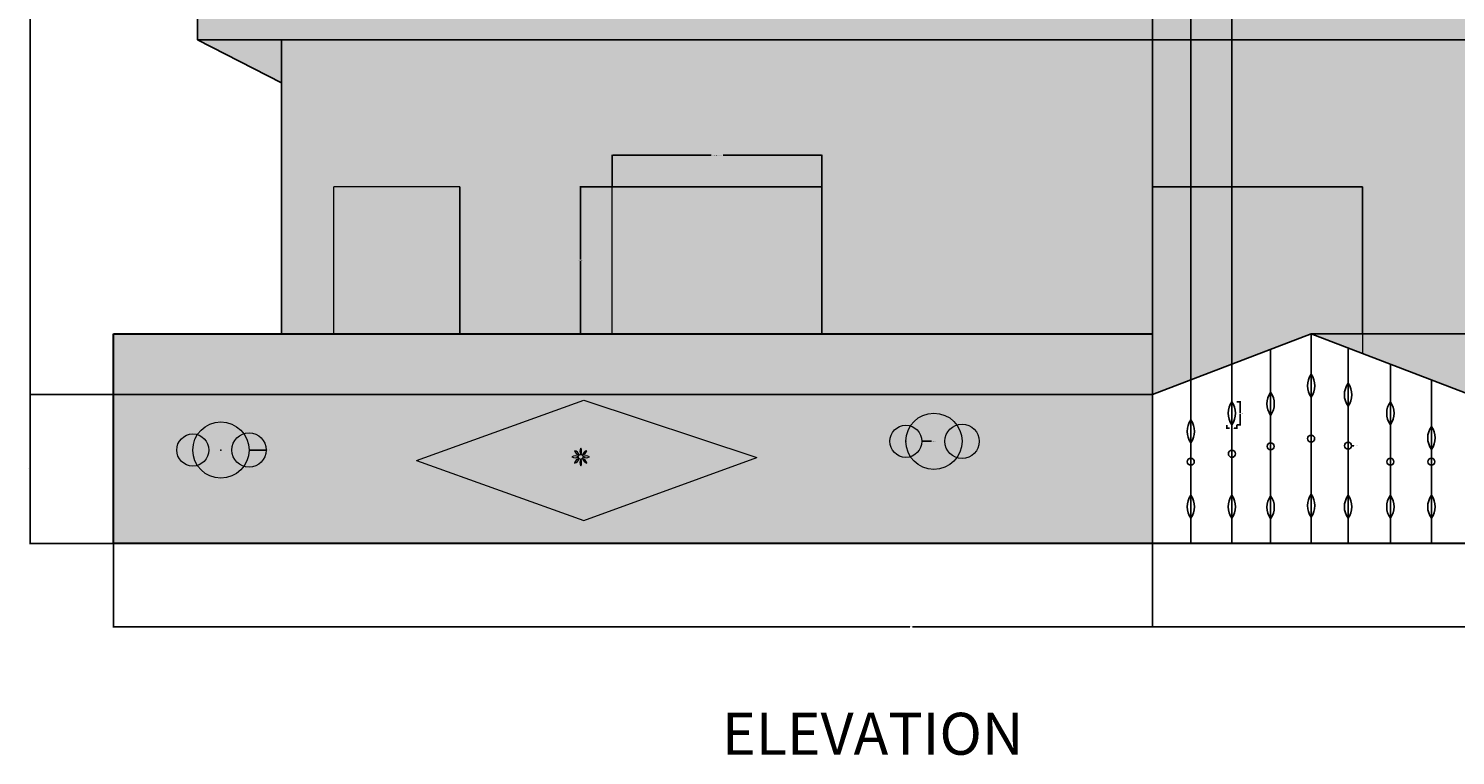
# Model space of a CAD drawing. Units: inches. Extents: x -43 to 1296, y -568 to 542.
# Tile 5 of 14: x -43 to 364, y 128 to 336. Entities that reach past the tile are written whole.
import ezdxf

# ---------------------------------------------------------------- set-up
doc = ezdxf.new("R2010")
doc.units = ezdxf.units.IN
doc.header["$MEASUREMENT"] = 0
for name, color, linetype, lineweight in [('A-ANNO-DIMS', 2, 'Continuous', 18), ('A-ANNO-TEXT', 7, 'Continuous', 18), ('A-DOOR', 3, 'Continuous', 18), ('A-ELEV', 7, 'Continuous', 25), ('A-ELEV-OPEN-PATT', 13, 'Continuous', 13), ('A-ELEV-TRIM', 7, 'Continuous', 18), ('A-ELEV-TRIM-PATT', 4, 'Continuous', 13), ('A-GLAZ-ELEV', 4, 'Continuous', 18), ('A-SITE-GATE', 7, 'Continuous', 25), ('A-SITE-WALL', 7, 'Continuous', 30), ('A-SITE-WALL-PATT', 142, 'Continuous', 13)]:
    doc.layers.add(name, color=color, linetype=linetype, lineweight=lineweight)
doc.layers.add('A-ELEV-BAND-PATT', color=30, linetype='Continuous', lineweight=13, true_color=0xf8991e)
doc.layers.add('A-ELEV-WALL-PATT', color=31, linetype='Continuous', lineweight=13, true_color=0xfecc66)
doc.styles.get("Standard").update_dxf_attribs({"font": 'arial.ttf'})
doc.dimstyles.get("Standard").update_dxf_attribs({"dimtxt": 0.18, "dimasz": 0.18, "dimexe": 0.18, "dimexo": 0.0625, "dimgap": 0.09, "dimtad": 0, "dimtih": 1, "dimtoh": 1, "dimdec": 0, "dimzin": 0, "dimdsep": 46, "dimlunit": 3, "dimtxsty": 'Standard', "dimcen": 0.09, "dimadec": 0, "dimazin": 0, "dimtfac": 1, "dimtdec": 0, "dimtofl": 0, "dimtmove": 0, "dimatfit": 3, "dimfxl": 1, "dimtolj": 1, "dimtzin": 0, "dimarcsym": 0})

# ---------------------------------------------------------------- blocks, each defined once
blk = doc.blocks.new('*U7')
for centre, start, end in [((1.42, 0), 147.6585, 212.3415), ((-1.42, 0), 327.6585, 32.3415)]:
    blk.add_arc(centre, 1.68, start, end)
blk = doc.blocks.new('*U8')
at = {"layer": 'A-ELEV-TRIM', "color": 0, "linetype": 'ByBlock', "lineweight": -2, "transparency": 16777216}
for p, rotation in [((112.78, 213.05), 90), ((113.25, 214.18), 45), ((113.25, 211.91), 135), ((114.38, 211.44), 180), ((115.51, 214.18), 315), ((115.51, 211.91), 225), ((115.98, 213.05), 270)]:
    blk.add_blockref('*U7', p, dxfattribs=dict(at, rotation=rotation))
blk.add_blockref('*U7', (114.38, 214.65), dxfattribs=at)
blk = doc.blocks.new('GATE-PICKET-LEAF')
for centre, start, end in [((5.7, 3.3), 144.6886, 215.3114), ((-3.6, 3.3), 324.6886, 35.3114)]:
    blk.add_arc(centre, 5.7, start, end)
blk = doc.blocks.new('WIN-ELEV-60x42')
for p, q in [((60, 42), (0, 42)), ((0, 0), (0, 42)), ((60, 0), (60, 42))]:
    blk.add_line(p, q)
blk = doc.blocks.new('*D50')
at = {"layer": 'A-ANNO-DIMS', "color": 0, "lineweight": -2, "transparency": 16777216}
for p, q in [((301.95, 228.81), (303.06, 228.81)), ((302.88, 228.63), (302.88, 225.7)), ((302.88, 222.4), (302.88, 225.33)), ((301.95, 222.22), (303.06, 222.22))]:
    blk.add_line(p, q, dxfattribs=at)
at = {"layer": 'A-ANNO-DIMS', "color": 0, "transparency": 16777216}
for points in [[(302.85, 228.63), (302.91, 228.63), (302.88, 228.81)], [(302.85, 222.4), (302.91, 222.4), (302.88, 222.22)]]:
    blk.add_solid(points, dxfattribs=at)
at = {"layer": 'Defpoints', "color": 0, "transparency": 16777216}
for p in [(301.89, 228.81), (302.88, 228.81), (301.89, 222.22)]:
    blk.add_point(p, dxfattribs=at)
at = {"layer": 'A-ANNO-DIMS', "color": 0, "transparency": 16777216, "insert": (302.88, 225.52), "char_height": 0.18, "attachment_point": 5}
blk.add_mtext('\\A1;LEAF 0\'-6 1/2" TYP.', dxfattribs=at)
blk = doc.blocks.new('*D51')
at = {"layer": 'A-ANNO-DIMS', "color": 0, "lineweight": -2, "transparency": 16777216}
for p, q in [((299.09, 222.16), (299.09, 221.05)), ((299.27, 221.23), (299.85, 221.23)), ((301.71, 221.23), (301.13, 221.23)), ((301.89, 222.16), (301.89, 221.05))]:
    blk.add_line(p, q, dxfattribs=at)
at = {"layer": 'A-ANNO-DIMS', "color": 0, "transparency": 16777216}
for points in [[(299.27, 221.26), (299.27, 221.2), (299.09, 221.23)], [(301.71, 221.26), (301.71, 221.2), (301.89, 221.23)]]:
    blk.add_solid(points, dxfattribs=at)
at = {"layer": 'Defpoints', "color": 0, "transparency": 16777216}
for p in [(299.09, 222.22), (301.89, 222.22), (301.89, 221.23)]:
    blk.add_point(p, dxfattribs=at)
at = {"layer": 'A-ANNO-DIMS', "color": 0, "transparency": 16777216, "insert": (300.49, 221.23), "char_height": 0.18, "attachment_point": 5}
blk.add_mtext('\\A1;0\'-3" TYP.', dxfattribs=at)
blk = doc.blocks.new('*D54')
at = {"layer": 'A-ANNO-DIMS', "color": 0, "lineweight": -2, "transparency": 16777216}
for p, q in [((123.34, 290.35), (123.34, 299.47)), ((123.52, 299.29), (151.63, 299.29)), ((183.16, 299.29), (155.06, 299.29)), ((183.34, 290.35), (183.34, 299.47))]:
    blk.add_line(p, q, dxfattribs=at)
at = {"layer": 'A-ANNO-DIMS', "color": 0, "transparency": 16777216}
for points in [[(123.52, 299.32), (123.52, 299.26), (123.34, 299.29)], [(183.16, 299.32), (183.16, 299.26), (183.34, 299.29)]]:
    blk.add_solid(points, dxfattribs=at)
at = {"layer": 'Defpoints', "color": 0, "transparency": 16777216}
for p in [(183.34, 299.29), (123.34, 290.29), (183.34, 290.29)]:
    blk.add_point(p, dxfattribs=at)
at = {"layer": 'A-ANNO-DIMS', "color": 0, "transparency": 16777216, "insert": (153.34, 299.29), "char_height": 0.18, "attachment_point": 5}
blk.add_mtext('\\A1;LOWER WINDOW 5\'-0" TYP.', dxfattribs=at)
blk = doc.blocks.new('*D55')
at = {"layer": 'A-ANNO-DIMS', "color": 0, "lineweight": -2, "transparency": 16777216}
for p, q in [((123.28, 290.29), (114.16, 290.29)), ((114.34, 290.11), (114.34, 269.47)), ((114.34, 248.47), (114.34, 269.11)), ((123.28, 248.29), (114.16, 248.29))]:
    blk.add_line(p, q, dxfattribs=at)
at = {"layer": 'A-ANNO-DIMS', "color": 0, "transparency": 16777216}
for points in [[(114.31, 290.11), (114.37, 290.11), (114.34, 290.29)], [(114.31, 248.47), (114.37, 248.47), (114.34, 248.29)]]:
    blk.add_solid(points, dxfattribs=at)
at = {"layer": 'Defpoints', "color": 0, "transparency": 16777216}
for p in [(114.34, 290.29), (123.34, 290.29), (123.34, 248.29)]:
    blk.add_point(p, dxfattribs=at)
at = {"layer": 'A-ANNO-DIMS', "color": 0, "transparency": 16777216, "insert": (114.34, 269.29), "char_height": 0.18, "attachment_point": 5}
blk.add_mtext('\\A1;3\'-6" TYP.', dxfattribs=at)
blk = doc.blocks.new('*D60')
at = {"layer": 'A-ANNO-DIMS', "color": 0, "lineweight": -2, "transparency": 16777216}
for p, q in [((-19.16, 188.23), (-19.16, 164.31)), ((436.84, 188.23), (436.84, 164.31)), ((-18.98, 164.49), (208.44, 164.49)), ((436.66, 164.49), (209.24, 164.49))]:
    blk.add_line(p, q, dxfattribs=at)
at = {"layer": 'A-ANNO-DIMS', "color": 0, "transparency": 16777216}
for points in [[(-18.98, 164.52), (-18.98, 164.46), (-19.16, 164.49)], [(436.66, 164.52), (436.66, 164.46), (436.84, 164.49)]]:
    blk.add_solid(points, dxfattribs=at)
at = {"layer": 'Defpoints', "color": 0, "transparency": 16777216}
for p in [(-19.16, 188.29), (436.84, 188.29), (436.84, 164.49)]:
    blk.add_point(p, dxfattribs=at)
at = {"layer": 'A-ANNO-DIMS', "color": 0, "transparency": 16777216, "insert": (208.84, 164.49), "char_height": 0.18, "attachment_point": 5}
blk.add_mtext('\\A1;38\'-0"', dxfattribs=at)
blk = doc.blocks.new('*D61')
at = {"layer": 'A-ANNO-DIMS', "color": 0, "lineweight": -2, "transparency": 16777216}
for p, q in [((4.78, 518.29), (-43.14, 518.29)), ((-42.96, 518.11), (-42.96, 353.47)), ((-42.96, 188.47), (-42.96, 353.11)), ((-19.22, 188.29), (-43.14, 188.29))]:
    blk.add_line(p, q, dxfattribs=at)
at = {"layer": 'A-ANNO-DIMS', "color": 0, "transparency": 16777216}
for points in [[(-42.99, 518.11), (-42.93, 518.11), (-42.96, 518.29)], [(-42.99, 188.47), (-42.93, 188.47), (-42.96, 188.29)]]:
    blk.add_solid(points, dxfattribs=at)
at = {"layer": 'Defpoints', "color": 0, "transparency": 16777216}
for p in [(-42.96, 518.29), (4.84, 518.29), (-19.16, 188.29)]:
    blk.add_point(p, dxfattribs=at)
at = {"layer": 'A-ANNO-DIMS', "color": 0, "transparency": 16777216, "insert": (-42.96, 353.29), "char_height": 0.18, "attachment_point": 5}
blk.add_mtext('\\A1;27\'-6"', dxfattribs=at)
blk = doc.blocks.new('*D67')
at = {"layer": 'A-ANNO-DIMS', "color": 0, "lineweight": -2, "transparency": 16777216}
for p, q in [((277.84, 188.23), (277.84, 164.31)), ((368.43, 188.23), (368.43, 164.31)), ((278.02, 164.49), (322.6, 164.49)), ((368.25, 164.49), (323.68, 164.49))]:
    blk.add_line(p, q, dxfattribs=at)
at = {"layer": 'A-ANNO-DIMS', "color": 0, "transparency": 16777216}
for points in [[(278.02, 164.52), (278.02, 164.46), (277.84, 164.49)], [(368.25, 164.52), (368.25, 164.46), (368.43, 164.49)]]:
    blk.add_solid(points, dxfattribs=at)
at = {"layer": 'Defpoints', "color": 0, "transparency": 16777216}
for p in [(277.84, 188.29), (368.43, 188.29), (368.43, 164.49)]:
    blk.add_point(p, dxfattribs=at)
at = {"layer": 'A-ANNO-DIMS', "color": 0, "transparency": 16777216, "insert": (323.14, 164.49), "char_height": 0.18, "attachment_point": 5}
blk.add_mtext('\\A1;7\'-6 1/2"', dxfattribs=at)
blk = doc.blocks.new('*D68')
at = {"layer": 'A-ANNO-DIMS', "color": 0, "lineweight": -2, "transparency": 16777216}
for p, q in [((277.78, 230.87), (-43.14, 230.87)), ((-42.96, 230.69), (-42.96, 209.77)), ((-42.96, 188.47), (-42.96, 209.4)), ((277.78, 188.29), (-43.14, 188.29))]:
    blk.add_line(p, q, dxfattribs=at)
at = {"layer": 'A-ANNO-DIMS', "color": 0, "transparency": 16777216}
for points in [[(-42.99, 230.69), (-42.93, 230.69), (-42.96, 230.87)], [(-42.99, 188.47), (-42.93, 188.47), (-42.96, 188.29)]]:
    blk.add_solid(points, dxfattribs=at)
at = {"layer": 'Defpoints', "color": 0, "transparency": 16777216}
for p in [(277.84, 230.87), (-42.96, 188.29), (277.84, 188.29)]:
    blk.add_point(p, dxfattribs=at)
at = {"layer": 'A-ANNO-DIMS', "color": 0, "transparency": 16777216, "insert": (-42.96, 209.58), "char_height": 0.18, "attachment_point": 5}
blk.add_mtext('\\A1;3\'-6 1/2"', dxfattribs=at)
blk = doc.blocks.new('*D69')
at = {"layer": 'A-ANNO-DIMS', "color": 0, "lineweight": -2, "transparency": 16777216}
for p, q in [((323.2, 248.29), (460.82, 248.29)), ((460.64, 248.11), (460.64, 218.47)), ((460.64, 188.47), (460.64, 218.11)), ((368.5, 188.29), (460.82, 188.29))]:
    blk.add_line(p, q, dxfattribs=at)
at = {"layer": 'A-ANNO-DIMS', "color": 0, "transparency": 16777216}
for points in [[(460.61, 248.11), (460.67, 248.11), (460.64, 248.29)], [(460.61, 188.47), (460.67, 188.47), (460.64, 188.29)]]:
    blk.add_solid(points, dxfattribs=at)
at = {"layer": 'Defpoints', "color": 0, "transparency": 16777216}
for p in [(323.14, 248.29), (368.43, 188.29), (460.64, 188.29)]:
    blk.add_point(p, dxfattribs=at)
at = {"layer": 'A-ANNO-DIMS', "color": 0, "transparency": 16777216, "insert": (460.64, 218.29), "char_height": 0.18, "attachment_point": 5}
blk.add_mtext('\\A1;5\'-0"', dxfattribs=at)
blk = doc.blocks.new('*D70')
at = {"layer": 'A-ANNO-DIMS', "color": 0, "lineweight": -2, "transparency": 16777216}
for p, q in [((277.84, 188.35), (277.84, 542.27)), ((278.02, 542.09), (282.89, 542.09)), ((288.57, 542.09), (283.69, 542.09)), ((288.75, 188.35), (288.75, 542.27))]:
    blk.add_line(p, q, dxfattribs=at)
at = {"layer": 'A-ANNO-DIMS', "color": 0, "transparency": 16777216}
for points in [[(278.02, 542.12), (278.02, 542.06), (277.84, 542.09)], [(288.57, 542.12), (288.57, 542.06), (288.75, 542.09)]]:
    blk.add_solid(points, dxfattribs=at)
at = {"layer": 'Defpoints', "color": 0, "transparency": 16777216}
for p in [(288.75, 542.09), (277.84, 188.29), (288.75, 188.29)]:
    blk.add_point(p, dxfattribs=at)
at = {"layer": 'A-ANNO-DIMS', "color": 0, "transparency": 16777216, "insert": (283.29, 542.09), "char_height": 0.18, "attachment_point": 5}
blk.add_mtext('\\A1;0\'-11"', dxfattribs=at)
blk = doc.blocks.new('*D71')
at = {"layer": 'A-ANNO-DIMS', "color": 0, "lineweight": -2, "transparency": 16777216}
for p, q in [((288.75, 235.13), (288.75, 542.27)), ((288.93, 542.09), (294.01, 542.09)), ((300.31, 542.09), (295.23, 542.09)), ((300.49, 239.65), (300.49, 542.27))]:
    blk.add_line(p, q, dxfattribs=at)
at = {"layer": 'A-ANNO-DIMS', "color": 0, "transparency": 16777216}
for points in [[(288.93, 542.12), (288.93, 542.06), (288.75, 542.09)], [(300.31, 542.12), (300.31, 542.06), (300.49, 542.09)]]:
    blk.add_solid(points, dxfattribs=at)
at = {"layer": 'Defpoints', "color": 0, "transparency": 16777216}
for p in [(300.49, 542.09), (300.49, 239.58), (288.75, 235.07)]:
    blk.add_point(p, dxfattribs=at)
at = {"layer": 'A-ANNO-DIMS', "color": 0, "transparency": 16777216, "insert": (294.62, 542.09), "char_height": 0.18, "attachment_point": 5}
blk.add_mtext('\\A1;0\'-11 1/2"', dxfattribs=at)
blk = doc.blocks.new('*D98')
at = {"layer": 'A-ANNO-DIMS', "color": 0, "lineweight": -2, "transparency": 16777216}
for p, q in [((333.62, 216.26), (333.8, 216.26)), ((333.71, 216.17), (333.71, 216.35)), ((335.31, 216.25), (334.89, 216.25))]:
    blk.add_line(p, q, dxfattribs=at)
at = {"layer": 'A-ANNO-DIMS', "color": 0, "transparency": 16777216}
blk.add_solid([(334.89, 216.28), (334.89, 216.22), (334.71, 216.25)], dxfattribs=at)
at = {"layer": 'Defpoints', "color": 0, "transparency": 16777216}
for p in [(332.71, 216.27), (334.71, 216.25)]:
    blk.add_point(p, dxfattribs=at)
at = {"layer": 'A-ANNO-DIMS', "color": 0, "transparency": 16777216, "insert": (335.93, 216.25), "char_height": 0.18, "attachment_point": 5}
blk.add_mtext('\\A1;7X ∅0\'-2"', dxfattribs=at)
blk = doc.blocks.new('*D99')
at = {"layer": 'A-ANNO-DIMS', "color": 0, "lineweight": -2, "transparency": 16777216}
for p, q in [((11.46, 215.02), (11.64, 215.02)), ((11.55, 214.93), (11.55, 215.11)), ((24.41, 215.02), (19.77, 215.02))]:
    blk.add_line(p, q, dxfattribs=at)
at = {"layer": 'A-ANNO-DIMS', "color": 0, "transparency": 16777216}
blk.add_solid([(19.77, 215.05), (19.77, 214.99), (19.59, 215.02)], dxfattribs=at)
at = {"layer": 'Defpoints', "color": 0, "transparency": 16777216}
for p in [(3.51, 215.02), (19.59, 215.02)]:
    blk.add_point(p, dxfattribs=at)
at = {"layer": 'A-ANNO-DIMS', "color": 0, "transparency": 16777216, "insert": (25.03, 215.02), "char_height": 0.18, "attachment_point": 5}
blk.add_mtext('\\A1;3X ∅1\'-4"', dxfattribs=at)
blk = doc.blocks.new('*D101')
at = {"layer": 'A-ANNO-DIMS', "color": 0, "lineweight": -2, "transparency": 16777216}
for p, q in [((207.21, 217.51), (207.39, 217.51)), ((207.3, 217.42), (207.3, 217.6)), ((214.65, 217.51), (212.07, 217.51))]:
    blk.add_line(p, q, dxfattribs=at)
at = {"layer": 'A-ANNO-DIMS', "color": 0, "transparency": 16777216}
blk.add_solid([(212.07, 217.54), (212.07, 217.48), (211.89, 217.51)], dxfattribs=at)
at = {"layer": 'Defpoints', "color": 0, "transparency": 16777216}
for p in [(202.71, 217.51), (211.89, 217.51)]:
    blk.add_point(p, dxfattribs=at)
at = {"layer": 'A-ANNO-DIMS', "color": 0, "transparency": 16777216, "insert": (215.26, 217.51), "char_height": 0.18, "attachment_point": 5}
blk.add_mtext('\\A1;3X ∅0\'-9"', dxfattribs=at)

msp = doc.modelspace()

# ---------------------------------------------------------------- hatches: boundary and pattern name
at = {"layer": 'A-ELEV-BAND-PATT'}
h = msp.add_hatch(color=256, dxfattribs=at)
h.dxf.hatch_style = 1
h.paths.add_polyline_path([(28.84, 332.29), (4.84, 332.29), (28.84, 320)])
h.paths.add_polyline_path([(412.84, 332.29), (388.84, 332.29), (388.84, 323.84)])
h.paths.add_polyline_path([(1184.13, 416.59), (824.13, 416.59), (824.13, 410.59), (1184.13, 410.59)])
h.paths.add_polyline_path([(1184.13, 272.59), (824.13, 272.59), (824.13, 266.59), (1184.13, 266.59)])
h = msp.add_hatch(color=256, dxfattribs=at)
h.dxf.hatch_style = 1
h.paths.add_polyline_path([(412.84, 374.29), (4.84, 374.29), (4.84, 332.29), (412.84, 332.29)])
h.paths.add_polyline_path([(222.28, 353.73, -0.197856), (210.28, 353.73, -0.131652), (209.89, 352.27, -0.197856), (220.28, 346.27, -0.197856), (209.89, 352.27, -0.131652), (208.82, 351.2, -0.197856), (214.82, 340.81, -0.197856), (208.82, 351.2, -0.131652), (207.36, 350.81, -0.197856), (207.36, 338.81, -0.197856), (207.36, 350.81, -0.131652), (205.9, 351.2, -0.197856), (199.9, 340.81, -0.197856), (205.9, 351.2, -0.131652), (204.83, 352.27, -0.197856), (194.44, 346.27, -0.197856), (204.83, 352.27, -0.131652), (204.44, 353.73, -0.197856), (192.44, 353.73, -0.197856), (204.44, 353.73, -0.131652), (204.83, 355.19, -0.197856), (194.44, 361.19, -0.197856), (204.83, 355.19, -0.131652), (205.9, 356.25, -0.197856), (199.9, 366.65, -0.197856), (205.9, 356.25, -0.131652), (207.36, 356.65, -0.197856), (207.36, 368.65, -0.197856), (207.36, 356.65, -0.131652), (208.82, 356.25, -0.197856), (214.82, 366.65, -0.197856), (208.82, 356.25, -0.131652), (209.89, 355.19, -0.197856), (220.28, 361.19, -0.197856), (209.89, 355.19, -0.131652), (210.28, 353.73, -0.197856)], flags=16)
h.paths.add_polyline_path([(263.61, 353.73, -0.197856), (275.61, 353.73, -0.131652), (276, 355.19, -0.197856), (265.61, 361.19, -0.197856), (276, 355.19, -0.131652), (277.07, 356.25, -0.197856), (271.07, 366.65, -0.197856), (277.07, 356.25, -0.131652), (278.53, 356.65, -0.197856), (278.53, 368.65, -0.197856), (278.53, 356.65, -0.131652), (279.99, 356.25, -0.197856), (285.99, 366.65, -0.197856), (279.99, 356.25, -0.131652), (281.06, 355.19, -0.197856), (291.45, 361.19, -0.197856), (281.06, 355.19, -0.131652), (281.45, 353.73, -0.197856), (293.45, 353.73, -0.197856), (281.45, 353.73, -0.131652), (281.06, 352.27, -0.197856), (291.45, 346.27, -0.197856), (281.06, 352.27, -0.131652), (279.99, 351.2, -0.197856), (285.99, 340.81, -0.197856), (279.99, 351.2, -0.131652), (278.53, 350.81, -0.197856), (278.53, 338.81, -0.197856), (278.53, 350.81, -0.131652), (277.07, 351.2, -0.197856), (271.07, 340.81, -0.197856), (277.07, 351.2, -0.131652), (276, 352.27, -0.197856), (265.61, 346.27, -0.197856), (276, 352.27, -0.131652), (275.61, 353.73, -0.197856)], flags=16)
h.paths.add_polyline_path([(330.52, 353.73, -0.197856), (342.52, 353.73, -0.131652), (342.91, 355.19, -0.197856), (332.52, 361.19, -0.197856), (342.91, 355.19, -0.131652), (343.98, 356.25, -0.197856), (337.98, 366.65, -0.197856), (343.98, 356.25, -0.131652), (345.44, 356.65, -0.197856), (345.44, 368.65, -0.197856), (345.44, 356.65, -0.131652), (346.9, 356.25, -0.197856), (352.9, 366.65, -0.197856), (346.9, 356.25, -0.131652), (347.97, 355.19, -0.197856), (358.36, 361.19, -0.197856), (347.97, 355.19, -0.131652), (348.36, 353.73, -0.197856), (360.36, 353.73, -0.197856), (348.36, 353.73, -0.131652), (347.97, 352.27, -0.197856), (358.36, 346.27, -0.197856), (347.97, 352.27, -0.131652), (346.9, 351.2, -0.197856), (352.9, 340.81, -0.197856), (346.9, 351.2, -0.131652), (345.44, 350.81, -0.197856), (345.44, 338.81, -0.197856), (345.44, 350.81, -0.131652), (343.98, 351.2, -0.197856), (337.98, 340.81, -0.197856), (343.98, 351.2, -0.131652), (342.91, 352.27, -0.197856), (332.52, 346.27, -0.197856), (342.91, 352.27, -0.131652), (342.52, 353.73, -0.197856)], flags=16)
h.paths.add_polyline_path([(148.25, 353.73, -0.197856), (136.25, 353.73, -0.131652), (135.85, 352.27, -0.197856), (146.25, 346.27, -0.197856), (135.85, 352.27, -0.131652), (134.79, 351.2, -0.197856), (140.79, 340.81, -0.197856), (134.79, 351.2, -0.131652), (133.33, 350.81, -0.197856), (133.33, 338.81, -0.197856), (133.33, 350.81, -0.131652), (131.87, 351.2, -0.197856), (125.87, 340.81, -0.197856), (131.87, 351.2, -0.131652), (130.8, 352.27, -0.197856), (120.41, 346.27, -0.197856), (130.8, 352.27, -0.131652), (130.41, 353.73, -0.197856), (118.41, 353.73, -0.197856), (130.41, 353.73, -0.131652), (130.8, 355.19, -0.197856), (120.41, 361.19, -0.197856), (130.8, 355.19, -0.131652), (131.87, 356.25, -0.197856), (125.87, 366.65, -0.197856), (131.87, 356.25, -0.131652), (133.33, 356.65, -0.197856), (133.33, 368.65, -0.197856), (133.33, 356.65, -0.131652), (134.79, 356.25, -0.197856), (140.79, 366.65, -0.197856), (134.79, 356.25, -0.131652), (135.85, 355.19, -0.197856), (146.25, 361.19, -0.197856), (135.85, 355.19, -0.131652), (136.25, 353.73, -0.197856)], flags=16)
h.paths.add_polyline_path([(80.61, 353.73, -0.197856), (68.61, 353.73, -0.131652), (68.22, 352.27, -0.197856), (78.61, 346.27, -0.197856), (68.22, 352.27, -0.131652), (67.15, 351.2, -0.197856), (73.15, 340.81, -0.197856), (67.15, 351.2, -0.131652), (65.69, 350.81, -0.197856), (65.69, 338.81, -0.197856), (65.69, 350.81, -0.131652), (64.23, 351.2, -0.197856), (58.23, 340.81, -0.197856), (64.23, 351.2, -0.131652), (63.16, 352.27, -0.197856), (52.77, 346.27, -0.197856), (63.16, 352.27, -0.131652), (62.77, 353.73, -0.197856), (50.77, 353.73, -0.197856), (62.77, 353.73, -0.131652), (63.16, 355.19, -0.197856), (52.77, 361.19, -0.197856), (63.16, 355.19, -0.131652), (64.23, 356.25, -0.197856), (58.23, 366.65, -0.197856), (64.23, 356.25, -0.131652), (65.69, 356.65, -0.197856), (65.69, 368.65, -0.197856), (65.69, 356.65, -0.131652), (67.15, 356.25, -0.197856), (73.15, 366.65, -0.197856), (67.15, 356.25, -0.131652), (68.22, 355.19, -0.197856), (78.61, 361.19, -0.197856), (68.22, 355.19, -0.131652), (68.61, 353.73, -0.197856)], flags=16)
at = {"layer": 'A-ELEV-OPEN-PATT'}
h = msp.add_hatch(color=256, dxfattribs=at)
h.dxf.hatch_style = 1
h.paths.add_polyline_path([(79.84, 434.29), (43.84, 434.29), (43.84, 374.29), (79.84, 374.29)])
h.paths.add_polyline_path([(183.34, 434.29), (123.34, 434.29), (123.34, 386.29), (183.34, 386.29)])
h.paths.add_polyline_path([(337.84, 434.29), (277.84, 434.29), (277.84, 386.29), (337.84, 386.29)])
h.paths.add_polyline_path([(79.84, 290.29), (43.84, 290.29), (43.84, 248.29), (79.84, 248.29)])
h.paths.add_polyline_path([(183.34, 290.29), (123.34, 290.29), (123.34, 248.29), (183.34, 248.29)])
h.paths.add_polyline_path([(337.84, 290.29), (277.84, 290.29), (277.84, 248.29), (277.84, 230.87), (323.14, 248.29), (337.84, 242.64), (337.84, 248.29)])
h.paths.add_polyline_path([(1016.13, 374.59), (980.13, 374.59), (980.13, 290.59), (1016.13, 290.59)])
h.paths.add_polyline_path([(1016.13, 230.59), (980.13, 230.59), (980.13, 146.59), (1016.13, 146.59)])
h.paths.add_polyline_path([(833.13, 374.59), (824.13, 374.59), (824.13, 326.59), (833.13, 326.59)])
h.paths.add_polyline_path([(833.13, 230.59), (824.13, 230.59), (824.13, 182.59), (833.13, 182.59)])
at = {"layer": 'A-ELEV-TRIM-PATT'}
h = msp.add_hatch(color=256, dxfattribs=at)
h.dxf.hatch_style = 1
h.paths.add_polyline_path([(164.68, 212.9), (115.24, 229.23), (67.47, 212.06), (115.24, 194.9)])
h.paths.add_polyline_path([(116.88, 213.05, -0.289973), (115.08, 213.05, -0.198912), (114.88, 212.55, -0.289973), (116.15, 211.28, -0.289973), (114.88, 212.55, -0.198912), (114.38, 212.34, -0.289973), (114.38, 210.55, -0.289973), (114.38, 212.34, -0.198912), (113.88, 212.55, -0.289973), (112.61, 211.28, -0.289973), (113.88, 212.55, -0.198912), (113.68, 213.05, -0.289973), (111.88, 213.05, -0.289973), (113.68, 213.05, -0.198912), (113.88, 213.54, -0.289973), (112.61, 214.81, -0.289973), (113.88, 213.54, -0.198912), (114.38, 213.75, -0.289973), (114.38, 215.55, -0.289973), (114.38, 213.75, -0.198912), (114.88, 213.54, -0.289973), (116.15, 214.81, -0.289973), (114.88, 213.54, -0.198912), (115.08, 213.05, -0.289973)], flags=16)
h.paths.add_polyline_path([(218.46, 217.51, -0.325786), (221.87, 222.19, 0.526984), (208.61, 221.91, -0.331674), (211.89, 217.51, -0.331674), (208.61, 213.11, 0.526984), (221.87, 212.82, -0.325786)])
h.paths.add_polyline_path([(404.4, 217.51, -0.325786), (407.82, 222.19, 0.526984), (394.56, 221.91, -0.331674), (397.84, 217.51, -0.331674), (394.56, 213.11, 0.526984), (407.82, 212.82, -0.325786)])
h.paths.add_polyline_path([(14.67, 215.02, -0.325786), (18.08, 219.7, 0.526984), (4.82, 219.42, -0.331674), (8.11, 215.02, -0.331674), (4.82, 210.62, 0.526984), (18.08, 210.34, -0.325786)])
h = msp.add_hatch(color=256, dxfattribs=at)
h.dxf.hatch_style = 1
h.paths.add_polyline_path([(115.08, 213.05, 1), (113.68, 213.05, 1)])
h.paths.add_polyline_path([(114.38, 215.55, 0.289973), (114.38, 213.75, 0.289973)])
h.paths.add_polyline_path([(112.61, 214.81, 0.289973), (113.88, 213.54, 0.289973)])
h.paths.add_polyline_path([(113.68, 213.05, 0.289973), (111.88, 213.05, 0.289973)])
h.paths.add_polyline_path([(113.88, 212.55, 0.289973), (112.61, 211.28, 0.289973)])
h.paths.add_polyline_path([(114.38, 212.34, 0.289973), (114.38, 210.55, 0.289973)])
h.paths.add_polyline_path([(114.88, 212.55, 0.289973), (116.15, 211.28, 0.289973)])
h.paths.add_polyline_path([(115.08, 213.05, 0.289973), (116.88, 213.05, 0.289973)])
h.paths.add_polyline_path([(116.15, 214.81, 0.289973), (114.88, 213.54, 0.289973)])
h.paths.add_polyline_path([(8.11, 215.02, 0.331674), (4.82, 219.42, 0.145907), (3.51, 215.02, 0.145907), (4.82, 210.62, 0.331674)])
h.paths.add_polyline_path([(19.59, 215.02, 0.156779), (18.08, 219.7, 0.325786), (14.67, 215.02, 0.325786), (18.08, 210.34, 0.156779)])
h.paths.add_polyline_path([(18.08, 219.7, -0.156779), (19.59, 215.02, -0.156779), (18.08, 210.34, 0.508539), (24.51, 215.02, 0.508539)])
h.paths.add_polyline_path([(4.82, 219.42, 0.501869), (-1.08, 215.02, 0.501869), (4.82, 210.62, -0.145907), (3.51, 215.02, -0.145907)])
h.paths.add_polyline_path([(228.3, 217.51, 0.508539), (221.87, 222.19, -0.156779), (223.38, 217.51, -0.156779), (221.87, 212.82, 0.508539)])
h.paths.add_polyline_path([(223.38, 217.51, 0.156779), (221.87, 222.19, 0.325786), (218.46, 217.51, 0.325786), (221.87, 212.82, 0.156779)])
h.paths.add_polyline_path([(211.89, 217.51, 0.331674), (208.61, 221.91, 0.145907), (207.3, 217.51, 0.145907), (208.61, 213.11, 0.331674)])
h.paths.add_polyline_path([(208.61, 221.91, 0.501869), (202.71, 217.51, 0.501869), (208.61, 213.11, -0.145907), (207.3, 217.51, -0.145907)])
h.paths.add_polyline_path([(407.82, 222.19, -0.156779), (409.32, 217.51, -0.156779), (407.82, 212.82, 0.508539), (414.24, 217.51, 0.508539)])
h.paths.add_polyline_path([(393.25, 217.51, -0.145907), (394.56, 221.91, 0.501869), (388.65, 217.51, 0.501869), (394.56, 213.11, -0.145907)])
h.paths.add_polyline_path([(397.84, 217.51, 0.331674), (394.56, 221.91, 0.145907), (393.25, 217.51, 0.145907), (394.56, 213.11, 0.331674)])
h.paths.add_polyline_path([(409.32, 217.51, 0.156779), (407.82, 222.19, 0.325786), (404.4, 217.51, 0.325786), (407.82, 212.82, 0.156779)])
at = {"layer": 'A-ELEV-WALL-PATT'}
h = msp.add_hatch(color=256, dxfattribs=at)
h.dxf.hatch_style = 1
h.paths.add_polyline_path([(388.84, 332.29), (28.84, 332.29), (28.84, 248.29), (43.84, 248.29), (43.84, 290.29), (79.84, 290.29), (79.84, 248.29), (123.34, 248.29), (123.34, 290.29), (183.34, 290.29), (183.34, 248.29), (277.84, 248.29), (277.84, 290.29), (337.84, 290.29), (337.84, 248.29), (337.84, 242.64), (368.43, 230.87), (368.43, 248.29), (388.84, 248.29)])
at = {"layer": 'A-SITE-WALL-PATT'}
h = msp.add_hatch(color=256, dxfattribs=at)
h.dxf.hatch_style = 1
h.paths.add_polyline_path([(277.84, 248.29), (-19.16, 248.29), (-19.16, 188.29), (28.84, 188.29), (277.84, 188.29)])
h.paths.add_polyline_path([(115.24, 229.23), (164.68, 212.9), (115.24, 194.9), (67.47, 212.06)], flags=16)
h.paths.add_polyline_path([(112.61, 214.81, -0.289973), (113.88, 213.54, -0.198912), (114.38, 213.75, -0.289973), (114.38, 215.55, -0.289973), (114.38, 213.75, -0.198912), (114.88, 213.54, -0.289973), (116.15, 214.81, -0.289973), (114.88, 213.54, -0.198912), (115.08, 213.05, -0.289973), (116.88, 213.05, -0.289973), (115.08, 213.05, -0.198912), (114.88, 212.55, -0.289973), (116.15, 211.28, -0.289973), (114.88, 212.55, -0.198912), (114.38, 212.34, -0.289973), (114.38, 210.55, -0.289973), (114.38, 212.34, -0.198912), (113.88, 212.55, -0.289973), (112.61, 211.28, -0.289973), (113.88, 212.55, -0.198912), (113.68, 213.05, -0.289973), (111.88, 213.05, -0.289973), (113.68, 213.05, -0.198912), (113.88, 213.54, -0.289973)], flags=0)
h.paths.add_polyline_path([(24.51, 215.02, -0.508539), (18.08, 210.34, -0.526984), (4.82, 210.62, -0.501869), (-1.08, 215.02, -0.501869), (4.82, 219.42, -0.526984), (18.08, 219.7, -0.508539)], flags=16)
h.paths.add_polyline_path([(208.61, 221.91, -0.526984), (221.87, 222.19, -0.508539), (228.3, 217.51, -0.508539), (221.87, 212.82, -0.526984), (208.61, 213.11, -0.501869), (202.71, 217.51, -0.501869)], flags=16)
h.paths.add_polyline_path([(436.84, 248.29), (368.43, 248.29), (368.43, 188.29), (388.84, 188.29), (436.84, 188.29)])
h.paths.add_polyline_path([(394.56, 221.91, -0.526984), (407.82, 222.19, -0.508539), (414.24, 217.51, -0.508539), (407.82, 212.82, -0.526984), (394.56, 213.11, -0.501869), (388.65, 217.51, -0.501869)], flags=16)

# ---------------------------------------------------------------- linework, layer by layer
at = {"layer": 'A-DOOR'}
for p, q in [((43.84, 248.29), (43.84, 290.29)), ((79.84, 290.29), (43.84, 290.29)), ((79.84, 248.29), (79.84, 290.29))]:
    msp.add_line(p, q, dxfattribs=at)
for points in [[(43.84, 248.29), (43.84, 290.29)], [(79.84, 290.29), (79.84, 248.29)]]:
    msp.add_lwpolyline(points, dxfattribs=at)
at = {"layer": 'A-ELEV'}
for p, q in [((4.84, 332.29), (4.84, 374.29)), ((412.84, 332.29), (4.84, 332.29)), ((4.84, 332.29), (28.84, 320)), ((28.84, 248.29), (28.84, 332.29))]:
    msp.add_line(p, q, dxfattribs=at)
at = {"layer": 'A-ELEV-TRIM'}
for p, q in [((67.47, 212.06), (115.24, 229.23)), ((115.24, 229.23), (164.68, 212.9)), ((115.24, 194.9), (164.68, 212.9)), ((67.47, 212.06), (115.24, 194.9))]:
    msp.add_line(p, q, dxfattribs=at)
for centre, radius in [((215.34, 217.51), 8.04), ((11.55, 215.02), 8.04), ((207.3, 217.51), 4.59), ((223.38, 217.51), 4.92), ((3.51, 215.02), 4.59), ((19.59, 215.02), 4.92), ((114.38, 213.05), 0.703)]:
    msp.add_circle(centre, radius, dxfattribs=at)
at = {"layer": 'A-GLAZ-ELEV'}
msp.add_line((337.84, 248.29), (337.84, 242.64), dxfattribs=at)
for points in [[(123.34, 248.29), (123.34, 290.29), (183.34, 290.29), (183.34, 248.29)], [(277.84, 248.29), (277.84, 290.29), (337.84, 290.29), (337.84, 248.29)]]:
    msp.add_lwpolyline(points, dxfattribs=at)
at = {"layer": 'A-SITE-GATE'}
for p, q in [((277.84, 248.29), (277.84, 188.29)), ((323.14, 248.29), (277.84, 230.87)), ((323.14, 248.29), (368.43, 230.87)), ((323.14, 248.29), (323.14, 188.29)), ((311.57, 243.84), (311.57, 188.29)), ((333.71, 244.23), (333.71, 188.29)), ((300.49, 239.58), (300.49, 188.29)), ((345.79, 239.58), (345.79, 188.29)), ((288.75, 235.07), (288.75, 188.29)), ((357.53, 235.07), (357.53, 188.29))]:
    msp.add_line(p, q, dxfattribs=at)
for centre in [(311.57, 216.07), (323.14, 218.29), (333.71, 216.26), (288.75, 211.68), (300.49, 213.94), (345.79, 211.68), (357.53, 211.68)]:
    msp.add_circle(centre, 1, dxfattribs=at)
at = {"layer": 'A-SITE-WALL'}
for p, q in [((-19.16, 188.29), (-19.16, 248.29)), ((-19.16, 248.29), (277.84, 248.29)), ((28.84, 188.29), (-19.16, 188.29)), ((388.84, 188.29), (28.84, 188.29))]:
    msp.add_line(p, q, dxfattribs=at)

# ---------------------------------------------------------------- block references
at = {"layer": 'A-ELEV-TRIM'}
msp.add_blockref('*U8', (0, 0), dxfattribs=at)
at = {"layer": 'A-GLAZ-ELEV'}
for p in [(123.34, 248.29), (277.84, 248.29)]:
    msp.add_blockref('WIN-ELEV-60x42', p, dxfattribs=at)
at = {"layer": 'A-SITE-GATE'}
for p in [(322.09, 230.1), (332.66, 227.52), (299.44, 222.22), (310.52, 224.93), (344.74, 222.22), (287.7, 217.06), (356.48, 215.19), (287.7, 195.48), (299.44, 195.48), (310.52, 195.34), (322.09, 195.81), (332.66, 195.48), (344.74, 195.48), (356.48, 195.48)]:
    msp.add_blockref('GATE-PICKET-LEAF', p, dxfattribs=at)

# ---------------------------------------------------------------- texts
at = {"layer": 'A-ANNO-TEXT', "insert": (154.77, 139.88), "char_height": 12, "attachment_point": 1}
msp.add_mtext('ELEVATION', dxfattribs=at)

# ---------------------------------------------------------------- dimensions: what is measured, and where the dimension line sits
at = {"layer": 'A-ANNO-DIMS'}
for base, p1, p2, picture, middle in [((288.75, 542.09), (277.84, 188.29), (288.75, 188.29), '*D70', (283.29, 542.09)), ((300.49, 542.09), (288.75, 235.07), (300.49, 239.58), '*D71', (294.62, 542.09)), ((436.84, 164.49), (-19.16, 188.29), (436.84, 188.29), '*D60', (208.84, 164.49)), ((368.43, 164.49), (277.84, 188.29), (368.43, 188.29), '*D67', (323.14, 164.49))]:
    dim = msp.add_linear_dim(base=base, p1=p1, p2=p2, dimstyle='Standard', override={"dimdec": 1, "dimlfac": 1, "dimrnd": 0, "dimzin": 1, "dimdsep": 46, "dimlunit": 4, "dimfrac": 2}, dxfattribs=at)
    dim.commit()
    dim.dimension.update_dxf_attribs({"geometry": picture, "text_midpoint": middle})
for base, p1, p2, picture, middle in [((-42.96, 518.29), (-19.16, 188.29), (4.84, 518.29), '*D61', (-42.96, 353.29)), ((460.64, 188.29), (323.14, 248.29), (368.43, 188.29), '*D69', (460.64, 218.29)), ((-42.96, 188.29), (277.84, 230.87), (277.84, 188.29), '*D68', (-42.96, 209.58))]:
    dim = msp.add_linear_dim(base=base, p1=p1, p2=p2, angle=90, dimstyle='Standard', override={"dimdec": 1, "dimlfac": 1, "dimrnd": 0, "dimzin": 1, "dimdsep": 46, "dimlunit": 4, "dimfrac": 2}, dxfattribs=at)
    dim.commit()
    dim.dimension.update_dxf_attribs({"geometry": picture, "text_midpoint": middle})
for base, p1, p2, text, picture, middle in [((183.34, 299.29), (123.34, 290.29), (183.34, 290.29), 'LOWER WINDOW <> TYP.', '*D54', (153.34, 299.29)), ((301.89, 221.23), (299.09, 222.22), (301.89, 222.22), '<> TYP.', '*D51', (300.49, 221.23))]:
    dim = msp.add_linear_dim(base=base, p1=p1, p2=p2, text=text, dimstyle='Standard', override={"dimdec": 1, "dimlfac": 1, "dimrnd": 0, "dimzin": 1, "dimdsep": 46, "dimlunit": 4, "dimfrac": 2}, dxfattribs=at)
    dim.commit()
    dim.dimension.update_dxf_attribs({"geometry": picture, "text_midpoint": middle})
for base, p1, p2, text, picture, middle in [((114.34, 290.29), (123.34, 248.29), (123.34, 290.29), '<> TYP.', '*D55', (114.34, 269.29)), ((302.88, 228.81), (301.89, 222.22), (301.89, 228.81), 'LEAF <> TYP.', '*D50', (302.88, 225.52))]:
    dim = msp.add_linear_dim(base=base, p1=p1, p2=p2, angle=90, text=text, dimstyle='Standard', override={"dimdec": 1, "dimlfac": 1, "dimrnd": 0, "dimzin": 1, "dimdsep": 46, "dimlunit": 4, "dimfrac": 2}, dxfattribs=at)
    dim.commit()
    dim.dimension.update_dxf_attribs({"geometry": picture, "text_midpoint": middle})
for p1, p2, text, picture, middle in [((202.71, 217.51), (211.89, 217.51), '3X <>', '*D101', (214.65, 217.51)), ((332.71, 216.27), (334.71, 216.25), '7X <>', '*D98', (335.31, 216.25)), ((3.51, 215.02), (19.59, 215.02), '3X <>', '*D99', (24.41, 215.02))]:
    dim = msp.add_diameter_dim_2p(p1=p1, p2=p2, text=text, dimstyle='Standard', override={"dimdec": 1, "dimlfac": 1, "dimrnd": 0, "dimzin": 1, "dimdsep": 46, "dimlunit": 4, "dimfrac": 2}, dxfattribs=at)
    dim.commit()
    dim.dimension.update_dxf_attribs({"geometry": picture, "text_midpoint": middle, "dimtype": 163})

doc.saveas('drawing.dxf')
